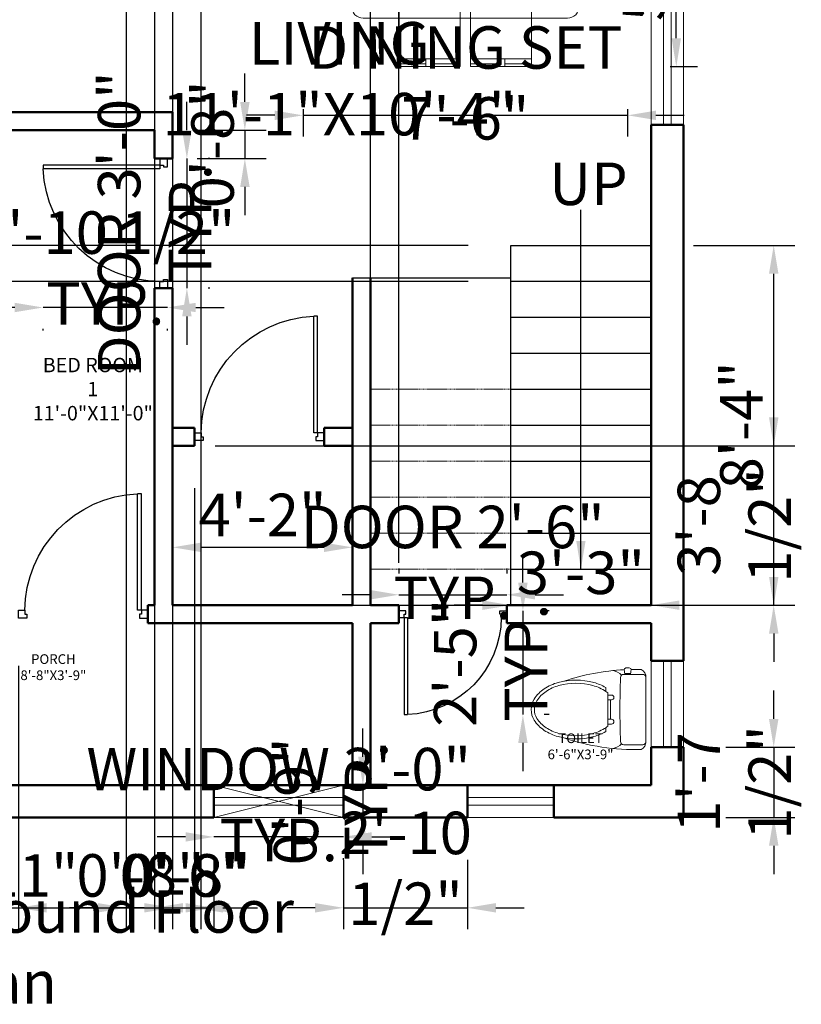
# Model space of a CAD drawing. Units: inches. Extents: x 314 to 688, y 344 to 882.
# Tile 2 of 3: x 471 to 688, y 344 to 618. Entities that reach past the tile are written whole.
import ezdxf

# ---------------------------------------------------------------- set-up
doc = ezdxf.new("R2010")
doc.units = ezdxf.units.IN
doc.header["$MEASUREMENT"] = 0
doc.linetypes.add('HIDDEN', pattern=[0.375, 0.25, -0.125])
for name, color, linetype, lineweight in [('A-ANNO-TEXT', 7, 'Continuous', 25), ('A-AREA-IDEN', 7, 'Continuous', 25), ('A-DOOR', 4, 'Continuous', 25), ('A-FLOR-FIXT', 9, 'Continuous', 18), ('A-FLOR-STRS', 7, 'Continuous', 25), ('A-FLOR-STRS-HIDN', 8, 'HIDDEN', 18), ('A-FURN', 8, 'Continuous', 18), ('WALL', 7, 'Continuous', 50), ('WINDOW', 2, 'Continuous', 18), ('YQ_DIM', 3, 'Continuous', 18)]:
    doc.layers.add(name, color=color, linetype=linetype, lineweight=lineweight)
doc.styles.add('YQ_DIM', font='SUPEROS.SHX', dxfattribs={"width": 0.8, "bigfont": 'HZDX.SHX'})
doc.dimstyles.new('yqi3_937', dxfattribs={"dimscale": 3.937008, "dimtxt": 3, "dimasz": 2, "dimexe": 1.5, "dimexo": 3, "dimgap": 0.5, "dimtad": 1, "dimdsep": 46, "dimlunit": 4, "dimtxsty": 'YQ_DIM', "dimcen": 0, "dimclrd": 256, "dimclre": 256, "dimclrt": 7, "dimadec": 1, "dimazin": 2, "dimtfac": 1, "dimtix": 1, "dimtmove": 2, "dimatfit": 2, "dimfxl": 1, "dimtolj": 1, "dimtzin": 0, "dimarcsym": 0})

# ---------------------------------------------------------------- blocks, each defined once
blk = doc.blocks.new('DR_D01')
for p, q in [((-0.45, 0.93), (-0.42, 0.93)), ((-0.45, 0.03), (-0.45, 0.93)), ((-0.42, 0.03), (-0.42, 0.93)), ((-0.5, 0.03), (-0.42, 0.03)), ((-0.5, 0.03), (-0.5, -0.03)), ((-0.45, 0.03), (-0.45, 0)), ((-0.45, 0), (-0.435, 0)), ((-0.435, 0), (-0.435, -0.03)), ((0.435, 0), (0.435, -0.03)), ((0.45, 0), (0.435, 0)), ((0.45, 0.03), (0.45, 0)), ((0.5, 0.03), (0.45, 0.03)), ((0.5, -0.03), (0.5, 0.03)), ((-0.435, -0.03), (-0.5, -0.03)), ((0.435, -0.03), (0.5, -0.03))]:
    blk.add_line(p, q)
blk.add_arc((-0.4602, 0.0206), 0.9103, 0.59152, 87.46644)
blk = doc.blocks.new('WD_WIN4')
for p, q in [((-0.5, 0.5), (0.5, 0.5)), ((-0.5, 0.12), (0.5, 0.12)), ((-0.5, -0.12), (0.5, -0.12)), ((-0.5, -0.5), (0.5, -0.5))]:
    blk.add_line(p, q)
blk = doc.blocks.new('*D7')
at = {"layer": 'Defpoints', "color": 0, "transparency": 16777216}
for p in [(513.29, 472.16), (563.29, 472.16), (563.29, 471.31)]:
    blk.add_point(p, dxfattribs=at)
at = {"layer": 'YQ_DIM', "color": 0, "lineweight": -2, "transparency": 16777216}
for p, q in [((521.17, 471.31), (555.42, 471.31)), ((513.29, 460.35), (513.29, 465.4)), ((563.29, 460.35), (563.29, 465.4))]:
    blk.add_line(p, q, dxfattribs=at)
at = {"layer": 'YQ_DIM', "color": 0, "transparency": 16777216}
for points in [[(521.17, 472.62), (521.17, 470), (513.29, 471.31)], [(555.42, 472.62), (555.42, 470), (563.29, 471.31)]]:
    blk.add_solid(points, dxfattribs=at)
at = {"layer": 'YQ_DIM', "color": 0, "transparency": 16777216, "insert": (538.29, 480.31), "char_height": 11.811, "attachment_point": 5, "style": 'YQ_DIM'}
blk.add_mtext('\\A1;4\'-2"', dxfattribs=at)
blk = doc.blocks.new('*D9')
at = {"layer": 'Defpoints', "color": 0, "transparency": 16777216}
for p in [(607.29, 460.65), (646.29, 460.65), (646.29, 455.23)]:
    blk.add_point(p, dxfattribs=at)
at = {"layer": 'YQ_DIM', "color": 0, "lineweight": -2, "transparency": 16777216}
for p, q in [((599.42, 455.23), (591.55, 455.23)), ((607.29, 455.23), (646.29, 455.23)), ((654.17, 455.23), (662.04, 455.23)), ((607.29, 448.84), (607.29, 449.33)), ((646.29, 448.84), (646.29, 449.33))]:
    blk.add_line(p, q, dxfattribs=at)
at = {"layer": 'YQ_DIM', "color": 0, "transparency": 16777216}
for points in [[(599.42, 456.54), (599.42, 453.92), (607.29, 455.23)], [(654.17, 456.54), (654.17, 453.92), (646.29, 455.23)]]:
    blk.add_solid(points, dxfattribs=at)
at = {"layer": 'YQ_DIM', "color": 0, "transparency": 16777216, "insert": (626.79, 464.23), "char_height": 11.811, "attachment_point": 5, "style": 'YQ_DIM'}
blk.add_mtext('\\A1;3\'-3"', dxfattribs=at)
blk = doc.blocks.new('yq_matong_01')
for p, q in [((0, 200.5), (0, -200.5)), ((20, 220.5), (138.8, 220.5)), ((252.5, 138), (252.5, 114.5)), ((215.8, 91), (238, 91)), ((238, 104.1), (238, -104.1)), ((215.8, 61), (238, 61)), ((223, 61), (223, -61)), ((215.8, -61), (238, -61)), ((215.8, -91), (238, -91)), ((252.5, -114.5), (252.5, -138)), ((20, -220.5), (138.8, -220.5)), ((97.4, -220.5), (97.4, -225.5)), ((97.4, -225.5), (131.6, -225.5)), ((131.6, -220.5), (131.6, -225.5))]:
    blk.add_line(p, q)
for centre, radius, start, end in [((54.8, 202.4), 54.8, 117.32201, 181.89921), ((63.9, -1165.4), 1416.8, 71.40679, 91.38565), ((20, 200.5), 20, 90, 180), ((138.8, 200.5), 20, 2.30634, 90), ((216.6, 161.2), 83.2, 95.49628, 139.93242), ((-4840.4, 0), 5003.3, 357.69366, 2.30634), ((406.6, -122.9), 283, 105.20877, 123.27785), ((406.6, -122.9), 303, 105.20877, 120.56985), ((439, -242.2), 426.7, 74.79123, 105.20877), ((439, -242.2), 406.7, 74.79123, 105.20877), ((471.4, -122.9), 283, 56.72215, 74.79123), ((471.4, -122.9), 303, 56.72215, 74.79123), ((520.9, -47.5), 212.8, 32.25649, 56.72215), ((215.8, 76), 15, 90, 270), ((357.1, -47.5), 192.8, 123.27785, 128.13838), ((520.9, -47.5), 192.8, 32.25649, 56.72215), ((596.2, 0), 123.8, 360, 32.25649), ((596.2, 0), 103.8, 360, 32.25649), ((215.8, -76), 15, 90, 270), ((520.9, 47.5), 192.8, 303.27785, 327.74351), ((596.2, 0), 103.8, 327.74351, 360), ((596.2, 0), 123.8, 327.74351, 360), ((357.1, 47.5), 192.8, 231.86162, 236.72215), ((406.6, 122.9), 283, 236.72215, 254.79123), ((471.4, 122.9), 283, 285.20877, 303.27785), ((520.9, 47.5), 212.8, 303.27785, 327.74351), ((63.9, 1165.4), 1416.8, 272.89667, 288.59321), ((406.6, 122.9), 303, 239.43015, 254.79123), ((439, 242.2), 426.7, 254.79123, 285.20877), ((439, 242.2), 406.7, 254.79123, 285.20877), ((471.4, 122.9), 303, 285.20877, 303.27785), ((51.3, -204.4), 51.4, 175.68696, 245.09182), ((20, -200.5), 20, 180, 270), ((156.6, -247.4), 63.1, 159.68336, 188.49388), ((72.4, -247.4), 63.1, 352.09441, 20.31664), ((138.8, -200.5), 20, 270, 357.69366), ((216.6, -161.2), 83.2, 220.06758, 264.50372), ((63.9, 1165.4), 1416.8, 268.61435, 271.20362), ((114.1, -225.6), 37, 237.52867, 304.27722)]:
    blk.add_arc(centre, radius, start, end)
blk = doc.blocks.new('East 1200 Sq.ft$0$din1')
for p, q in [((-487.5, 578.6), (-487.5, 807.1)), ((-487.5, 807.1), (-291.1, 807.1)), ((-291.1, 750), (-291.1, 807.1)), ((-291.1, 807.1), (-233.9, 807.1)), ((-233.9, 750), (-233.9, 807.1)), ((-233.9, 807.1), (-37.5, 807.1)), ((-37.5, 807.1), (-37.5, 578.6)), ((37.5, 807.1), (37.5, 578.6)), ((233.9, 807.1), (37.5, 807.1)), ((233.9, 750), (233.9, 807.1)), ((291.1, 807.1), (233.9, 807.1)), ((487.5, 807.1), (291.1, 807.1)), ((291.1, 750), (291.1, 807.1)), ((487.5, 578.6), (487.5, 807.1)), ((-487.5, 785.7), (-291.1, 785.7)), ((-487.5, 750), (-37.5, 750)), ((-233.9, 785.7), (-37.5, 785.7)), ((233.9, 785.7), (37.5, 785.7)), ((487.5, 750), (37.5, 750)), ((487.5, 785.7), (291.1, 785.7)), ((-966.1, 225), (-1194.6, 225)), ((-1194.6, 225), (-1194.6, 28.6)), ((-1173.2, 225), (-1173.2, 28.6)), ((-1137.5, 225), (-1137.5, -225)), ((966.1, 225), (1194.6, 225)), ((1137.5, 225), (1137.5, -225)), ((1173.2, 225), (1173.2, 28.6)), ((1194.6, 225), (1194.6, 28.6)), ((-1137.5, 28.6), (-1194.6, 28.6)), ((-1194.6, 28.6), (-1194.6, -28.6)), ((1137.5, 28.6), (1194.6, 28.6)), ((1194.6, 28.6), (1194.6, -28.6)), ((-1137.5, -28.6), (-1194.6, -28.6)), ((-1194.6, -28.6), (-1194.6, -225)), ((-1173.2, -28.6), (-1173.2, -225)), ((1137.5, -28.6), (1194.6, -28.6)), ((1173.2, -28.6), (1173.2, -225)), ((1194.6, -28.6), (1194.6, -225)), ((-1194.6, -225), (-966.1, -225)), ((1194.6, -225), (966.1, -225)), ((-487.5, -578.6), (-487.5, -807.1)), ((-37.5, -807.1), (-37.5, -578.6)), ((37.5, -807.1), (37.5, -578.6)), ((487.5, -578.6), (487.5, -807.1)), ((-487.5, -750), (-37.5, -750)), ((-487.5, -785.7), (-291.1, -785.7)), ((-291.1, -750), (-291.1, -807.1)), ((-233.9, -750), (-233.9, -807.1)), ((-233.9, -785.7), (-37.5, -785.7)), ((487.5, -750), (37.5, -750)), ((233.9, -785.7), (37.5, -785.7)), ((233.9, -750), (233.9, -807.1)), ((291.1, -750), (291.1, -807.1)), ((487.5, -785.7), (291.1, -785.7)), ((-487.5, -807.1), (-291.1, -807.1)), ((-291.1, -807.1), (-233.9, -807.1)), ((-233.9, -807.1), (-37.5, -807.1)), ((233.9, -807.1), (37.5, -807.1)), ((291.1, -807.1), (233.9, -807.1)), ((487.5, -807.1), (291.1, -807.1))]:
    blk.add_line(p, q)
for points in [[(-37.5, 578.6), (-37.5, 342.9, -0.414214), (-80.4, 300), (-444.6, 300, -0.414214), (-487.5, 342.9), (-487.5, 578.6)], [(37.5, 578.6), (37.5, 342.9, 0.414214), (80.4, 300), (444.6, 300, 0.414214), (487.5, 342.9), (487.5, 578.6)], [(-966.1, -225), (-730.4, -225, 0.414214), (-687.5, -182.1), (-687.5, 182.1, 0.414214), (-730.4, 225), (-966.1, 225)], [(966.1, -225), (730.4, -225, -0.414214), (687.5, -182.1), (687.5, 182.1, -0.414214), (730.4, 225), (966.1, 225)], [(-37.5, -578.6), (-37.5, -342.9, 0.414214), (-80.4, -300), (-444.6, -300, 0.414214), (-487.5, -342.9), (-487.5, -578.6)], [(37.5, -578.6), (37.5, -342.9, -0.414214), (80.4, -300), (444.6, -300, -0.414214), (487.5, -342.9), (487.5, -578.6)]]:
    blk.add_lwpolyline(points, format="xyb")
blk.add_lwpolyline([(751.8, -450), (-751.8, -450, -0.414214), (-837.5, -364.3), (-837.5, 364.3, -0.414214), (-751.8, 450), (751.8, 450, -0.414214), (837.5, 364.3), (837.5, -364.3, -0.414214)], format="xyb", close=True)
blk = doc.blocks.new('*D20')
at = {"layer": 'Defpoints', "color": 0, "transparency": 16777216}
for p in [(524.79, 396.23), (560.79, 396.23), (524.79, 390.83)]:
    blk.add_point(p, dxfattribs=at)
at = {"layer": 'YQ_DIM', "lineweight": -2, "transparency": 16777216}
for p, q in [((516.92, 390.83), (509.05, 390.83)), ((560.79, 390.83), (524.79, 390.83)), ((568.67, 390.83), (576.54, 390.83)), ((524.79, 384.42), (524.79, 384.93)), ((560.79, 384.42), (560.79, 384.93))]:
    blk.add_line(p, q, dxfattribs=at)
at = {"layer": 'YQ_DIM', "transparency": 16777216}
for points in [[(516.92, 392.14), (516.92, 389.52), (524.79, 390.83)], [(568.67, 392.14), (568.67, 389.52), (560.79, 390.83)]]:
    blk.add_solid(points, dxfattribs=at)
at = {"layer": 'YQ_DIM', "color": 7, "transparency": 16777216, "insert": (542.79, 399.83), "char_height": 11.811, "attachment_point": 5, "style": 'YQ_DIM'}
blk.add_mtext('\\A1;WINDOW 3\'-0" TYP.', dxfattribs=at)
blk = doc.blocks.new('*D21')
at = {"layer": 'Defpoints', "color": 0, "transparency": 16777216}
for p in [(560.79, 405.23), (560.79, 396.23), (566.19, 396.23)]:
    blk.add_point(p, dxfattribs=at)
at = {"layer": 'YQ_DIM', "lineweight": -2, "transparency": 16777216}
for p, q in [((566.19, 413.11), (566.19, 420.98)), ((566.19, 405.23), (566.19, 396.23)), ((572.6, 405.23), (572.1, 405.23)), ((572.6, 396.23), (572.1, 396.23)), ((566.19, 388.36), (566.19, 380.48))]:
    blk.add_line(p, q, dxfattribs=at)
at = {"layer": 'YQ_DIM', "transparency": 16777216}
for points in [[(564.88, 413.11), (567.51, 413.11), (566.19, 405.23)], [(564.88, 388.36), (567.51, 388.36), (566.19, 396.23)]]:
    blk.add_solid(points, dxfattribs=at)
at = {"layer": 'YQ_DIM', "color": 7, "transparency": 16777216, "insert": (557.2, 400.73), "char_height": 11.811, "attachment_point": 5, "rotation": 90, "style": 'YQ_DIM'}
blk.add_mtext('\\A1;0\'-9" TYP.', dxfattribs=at)
blk = doc.blocks.new('*D22')
at = {"layer": 'Defpoints', "color": 0, "transparency": 16777216}
for p in [(606.17, 458.13), (576.17, 453.63), (606.17, 453.63)]:
    blk.add_point(p, dxfattribs=at)
at = {"layer": 'YQ_DIM', "lineweight": -2, "transparency": 16777216}
for p, q in [((576.17, 465.44), (576.17, 464.04)), ((606.17, 465.44), (606.17, 464.04)), ((568.29, 458.13), (560.42, 458.13)), ((576.17, 458.13), (606.17, 458.13)), ((614.04, 458.13), (621.92, 458.13))]:
    blk.add_line(p, q, dxfattribs=at)
at = {"layer": 'YQ_DIM', "transparency": 16777216}
for points in [[(568.29, 459.44), (568.29, 456.82), (576.17, 458.13)], [(614.04, 459.44), (614.04, 456.82), (606.17, 458.13)]]:
    blk.add_solid(points, dxfattribs=at)
at = {"layer": 'YQ_DIM', "color": 7, "transparency": 16777216, "insert": (591.17, 467.13), "char_height": 11.811, "attachment_point": 5, "style": 'YQ_DIM'}
blk.add_mtext('\\A1;DOOR 2\'-6" TYP.', dxfattribs=at)
blk = doc.blocks.new('*D23')
at = {"layer": 'Defpoints', "color": 0, "transparency": 16777216}
for p in [(606.17, 453.63), (606.17, 424.83), (610.67, 424.83)]:
    blk.add_point(p, dxfattribs=at)
at = {"layer": 'YQ_DIM', "lineweight": -2, "transparency": 16777216}
for p, q in [((610.67, 461.51), (610.67, 469.38)), ((610.67, 453.63), (610.67, 424.83)), ((617.98, 453.63), (616.57, 453.63)), ((617.98, 424.83), (616.57, 424.83)), ((610.67, 416.96), (610.67, 409.08))]:
    blk.add_line(p, q, dxfattribs=at)
at = {"layer": 'YQ_DIM', "transparency": 16777216}
for points in [[(609.36, 461.51), (611.98, 461.51), (610.67, 453.63)], [(609.36, 416.96), (611.98, 416.96), (610.67, 424.83)]]:
    blk.add_solid(points, dxfattribs=at)
at = {"layer": 'YQ_DIM', "color": 7, "transparency": 16777216, "insert": (601.67, 439.23), "char_height": 11.811, "attachment_point": 5, "rotation": 90, "style": 'YQ_DIM'}
blk.add_mtext('\\A1;2\'-5" TYP.', dxfattribs=at)
blk = doc.blocks.new('*D24')
at = {"layer": 'Defpoints', "color": 0, "transparency": 16777216}
for p in [(511.87, 579.36), (511.87, 543.36), (517.27, 543.36)]:
    blk.add_point(p, dxfattribs=at)
at = {"layer": 'YQ_DIM', "lineweight": -2, "transparency": 16777216}
for p, q in [((517.27, 587.23), (517.27, 595.11)), ((517.27, 579.36), (517.27, 543.36)), ((523.68, 579.36), (523.18, 579.36)), ((523.68, 543.36), (523.18, 543.36)), ((517.27, 535.48), (517.27, 527.61))]:
    blk.add_line(p, q, dxfattribs=at)
at = {"layer": 'YQ_DIM', "transparency": 16777216}
for points in [[(515.96, 587.23), (518.59, 587.23), (517.27, 579.36)], [(515.96, 535.48), (518.59, 535.48), (517.27, 543.36)]]:
    blk.add_solid(points, dxfattribs=at)
at = {"layer": 'YQ_DIM', "color": 7, "transparency": 16777216, "insert": (508.28, 561.36), "char_height": 11.811, "attachment_point": 5, "rotation": 90, "style": 'YQ_DIM'}
blk.add_mtext('\\A1;DOOR 3\'-0" TYP.', dxfattribs=at)
blk = doc.blocks.new('*D25')
at = {"layer": 'Defpoints', "color": 0, "transparency": 16777216}
for p in [(477.31, 543.36), (511.87, 543.36), (477.31, 537.96)]:
    blk.add_point(p, dxfattribs=at)
at = {"layer": 'YQ_DIM', "lineweight": -2, "transparency": 16777216}
for p, q in [((469.44, 537.96), (461.57, 537.96)), ((511.87, 537.96), (477.31, 537.96)), ((519.75, 537.96), (527.62, 537.96)), ((477.31, 531.55), (477.31, 532.05)), ((511.87, 531.55), (511.87, 532.05))]:
    blk.add_line(p, q, dxfattribs=at)
at = {"layer": 'YQ_DIM', "transparency": 16777216}
for points in [[(469.44, 539.27), (469.44, 536.65), (477.31, 537.96)], [(519.75, 539.27), (519.75, 536.65), (511.87, 537.96)]]:
    blk.add_solid(points, dxfattribs=at)
at = {"layer": 'YQ_DIM', "color": 7, "transparency": 16777216, "insert": (494.59, 548.93), "char_height": 11.811, "attachment_point": 5, "style": 'YQ_DIM'}
blk.add_mtext('\\A1;2\'-10 1/2" TYP.', dxfattribs=at)
blk = doc.blocks.new('*D34')
at = {"layer": 'Defpoints', "color": 0, "transparency": 16777216}
for p in [(549.56, 604.9), (639.78, 604.9), (639.78, 591.37)]:
    blk.add_point(p, dxfattribs=at)
at = {"layer": 'YQ_DIM', "lineweight": -2, "transparency": 16777216}
for p, q in [((541.68, 591.37), (533.81, 591.37)), ((549.56, 593.09), (549.56, 585.46)), ((549.56, 591.37), (639.78, 591.37)), ((639.78, 593.09), (639.78, 585.46)), ((647.65, 591.37), (655.53, 591.37))]:
    blk.add_line(p, q, dxfattribs=at)
at = {"layer": 'YQ_DIM', "transparency": 16777216}
for points in [[(541.68, 592.68), (541.68, 590.05), (549.56, 591.37)], [(647.65, 592.68), (647.65, 590.05), (639.78, 591.37)]]:
    blk.add_solid(points, dxfattribs=at)
at = {"layer": 'YQ_DIM', "color": 7, "transparency": 16777216, "insert": (594.67, 600.37), "char_height": 11.811, "attachment_point": 5, "style": 'YQ_DIM'}
blk.add_mtext('\\A1;DINING SET 7\'-6"', dxfattribs=at)
blk = doc.blocks.new('*D35')
at = {"layer": 'Defpoints', "color": 0, "transparency": 16777216}
for p in [(639.78, 665.86), (653.31, 665.86), (639.78, 604.9)]:
    blk.add_point(p, dxfattribs=at)
at = {"layer": 'YQ_DIM', "lineweight": -2, "transparency": 16777216}
for p, q in [((651.59, 665.86), (659.22, 665.86)), ((653.31, 612.77), (653.31, 657.98)), ((651.59, 604.9), (659.22, 604.9))]:
    blk.add_line(p, q, dxfattribs=at)
at = {"layer": 'YQ_DIM', "transparency": 16777216}
for points in [[(652, 657.98), (654.62, 657.98), (653.31, 665.86)], [(652, 612.77), (654.62, 612.77), (653.31, 604.9)]]:
    blk.add_solid(points, dxfattribs=at)
at = {"layer": 'YQ_DIM', "color": 7, "transparency": 16777216, "insert": (644.31, 635.38), "char_height": 11.811, "attachment_point": 5, "rotation": 90, "style": 'YQ_DIM'}
blk.add_mtext('\\A1;5\'-1"', dxfattribs=at)
blk = doc.blocks.new('*D38')
at = {"layer": 'Defpoints', "color": 0, "transparency": 16777216}
for p in [(655.29, 415.73), (655.29, 396.23), (680.39, 396.23)]:
    blk.add_point(p, dxfattribs=at)
at = {"layer": 'YQ_DIM', "lineweight": -2, "transparency": 16777216}
for p, q in [((680.39, 423.61), (680.39, 431.48)), ((667.1, 415.73), (686.3, 415.73)), ((680.39, 415.73), (680.39, 396.23)), ((667.1, 396.23), (686.3, 396.23)), ((680.39, 388.36), (680.39, 380.48))]:
    blk.add_line(p, q, dxfattribs=at)
at = {"layer": 'YQ_DIM', "transparency": 16777216}
for points in [[(679.08, 423.61), (681.71, 423.61), (680.39, 415.73)], [(679.08, 388.36), (681.71, 388.36), (680.39, 396.23)]]:
    blk.add_solid(points, dxfattribs=at)
at = {"layer": 'YQ_DIM', "color": 7, "transparency": 16777216, "insert": (669.43, 405.98), "char_height": 11.811, "attachment_point": 5, "rotation": 90, "style": 'YQ_DIM'}
blk.add_mtext('\\A1;1\'-7 1/2"', dxfattribs=at)
blk = doc.blocks.new('*D39')
at = {"layer": 'Defpoints', "color": 0, "transparency": 16777216}
for p in [(646.29, 555.23), (680.39, 555.23), (646.29, 455.23)]:
    blk.add_point(p, dxfattribs=at)
at = {"layer": 'YQ_DIM', "lineweight": -2, "transparency": 16777216}
for p, q in [((658.1, 555.23), (686.3, 555.23)), ((680.39, 463.11), (680.39, 547.36)), ((658.1, 455.23), (686.3, 455.23))]:
    blk.add_line(p, q, dxfattribs=at)
at = {"layer": 'YQ_DIM', "transparency": 16777216}
for points in [[(679.08, 547.36), (681.71, 547.36), (680.39, 555.23)], [(679.08, 463.11), (681.71, 463.11), (680.39, 455.23)]]:
    blk.add_solid(points, dxfattribs=at)
at = {"layer": 'YQ_DIM', "color": 7, "transparency": 16777216, "insert": (671.4, 505.23), "char_height": 11.811, "attachment_point": 5, "rotation": 90, "style": 'YQ_DIM'}
blk.add_mtext('\\A1;8\'-4"', dxfattribs=at)
blk = doc.blocks.new('*D40')
at = {"layer": 'Defpoints', "color": 0, "transparency": 16777216}
for p in [(342.19, 555.23), (607.29, 555.23), (607.29, 545.23)]:
    blk.add_point(p, dxfattribs=at)
at = {"layer": 'YQ_DIM', "lineweight": -2, "transparency": 16777216}
for p, q in [((342.19, 563.11), (342.19, 570.98)), ((595.48, 555.23), (336.29, 555.23)), ((342.19, 545.23), (342.19, 555.23)), ((595.48, 545.23), (336.29, 545.23)), ((342.19, 537.36), (342.19, 529.48))]:
    blk.add_line(p, q, dxfattribs=at)
at = {"layer": 'YQ_DIM', "transparency": 16777216}
for points in [[(340.88, 563.11), (343.51, 563.11), (342.19, 555.23)], [(340.88, 537.36), (343.51, 537.36), (342.19, 545.23)]]:
    blk.add_solid(points, dxfattribs=at)
at = {"layer": 'YQ_DIM', "color": 7, "transparency": 16777216, "insert": (333.2, 550.23), "char_height": 11.811, "attachment_point": 5, "rotation": 90, "style": 'YQ_DIM'}
blk.add_mtext('\\A1;0\'-10"', dxfattribs=at)
blk = doc.blocks.new('*D46')
at = {"layer": 'Defpoints', "color": 0, "transparency": 16777216}
for p in [(367.29, 396.23), (524.79, 396.23), (524.79, 371.13)]:
    blk.add_point(p, dxfattribs=at)
at = {"layer": 'YQ_DIM', "lineweight": -2, "transparency": 16777216}
for p, q in [((367.29, 384.42), (367.29, 365.23)), ((524.79, 384.42), (524.79, 365.23)), ((375.17, 371.13), (516.92, 371.13))]:
    blk.add_line(p, q, dxfattribs=at)
at = {"layer": 'YQ_DIM', "transparency": 16777216}
for points in [[(375.17, 372.44), (375.17, 369.82), (367.29, 371.13)], [(516.92, 372.44), (516.92, 369.82), (524.79, 371.13)]]:
    blk.add_solid(points, dxfattribs=at)
at = {"layer": 'YQ_DIM', "color": 7, "transparency": 16777216, "insert": (446.04, 382.1), "char_height": 11.811, "attachment_point": 5, "style": 'YQ_DIM'}
blk.add_mtext('\\A1;13\'-1 1/2"', dxfattribs=at)
blk = doc.blocks.new('*D47')
at = {"layer": 'Defpoints', "color": 0, "transparency": 16777216}
for p in [(560.79, 396.23), (595.29, 396.23), (595.29, 371.13)]:
    blk.add_point(p, dxfattribs=at)
at = {"layer": 'YQ_DIM', "lineweight": -2, "transparency": 16777216}
for p, q in [((560.79, 384.42), (560.79, 365.23)), ((595.29, 384.42), (595.29, 365.23)), ((552.92, 371.13), (545.05, 371.13)), ((560.79, 371.13), (595.29, 371.13)), ((603.17, 371.13), (611.04, 371.13))]:
    blk.add_line(p, q, dxfattribs=at)
at = {"layer": 'YQ_DIM', "transparency": 16777216}
for points in [[(552.92, 372.44), (552.92, 369.82), (560.79, 371.13)], [(603.17, 372.44), (603.17, 369.82), (595.29, 371.13)]]:
    blk.add_solid(points, dxfattribs=at)
at = {"layer": 'YQ_DIM', "color": 7, "transparency": 16777216, "insert": (578.04, 382.1), "char_height": 11.811, "attachment_point": 5, "style": 'YQ_DIM'}
blk.add_mtext('\\A1;2\'-10 1/2"', dxfattribs=at)
blk = doc.blocks.new('*D48')
at = {"layer": 'Defpoints', "color": 0, "transparency": 16777216}
for p in [(513.29, 499.55), (680.39, 499.55), (513.29, 455.23)]:
    blk.add_point(p, dxfattribs=at)
at = {"layer": 'YQ_DIM', "lineweight": -2, "transparency": 16777216}
for p, q in [((680.39, 507.42), (680.39, 515.3)), ((525.1, 499.55), (686.3, 499.55)), ((680.39, 455.23), (680.39, 499.55)), ((525.1, 455.23), (686.3, 455.23)), ((680.39, 447.36), (680.39, 439.48))]:
    blk.add_line(p, q, dxfattribs=at)
at = {"layer": 'YQ_DIM', "transparency": 16777216}
for points in [[(679.08, 507.42), (681.71, 507.42), (680.39, 499.55)], [(679.08, 447.36), (681.71, 447.36), (680.39, 455.23)]]:
    blk.add_solid(points, dxfattribs=at)
at = {"layer": 'YQ_DIM', "color": 7, "transparency": 16777216, "insert": (669.43, 477.39), "char_height": 11.811, "attachment_point": 5, "rotation": 90, "style": 'YQ_DIM'}
blk.add_mtext('\\A1;3\'-8 1/2"', dxfattribs=at)
blk = doc.blocks.new('*D49')
at = {"layer": 'Defpoints', "color": 0, "transparency": 16777216}
for p in [(508.29, 675.23), (500.42, 670.23), (508.29, 371.13)]:
    blk.add_point(p, dxfattribs=at)
at = {"layer": 'YQ_DIM', "lineweight": -2, "transparency": 16777216}
for p, q in [((508.29, 663.42), (508.29, 365.23)), ((500.42, 658.42), (500.42, 365.23)), ((492.55, 371.13), (484.67, 371.13)), ((500.42, 371.13), (508.29, 371.13)), ((516.17, 371.13), (524.04, 371.13))]:
    blk.add_line(p, q, dxfattribs=at)
at = {"layer": 'YQ_DIM', "transparency": 16777216}
for points in [[(492.55, 372.44), (492.55, 369.82), (500.42, 371.13)], [(516.17, 372.44), (516.17, 369.82), (508.29, 371.13)]]:
    blk.add_solid(points, dxfattribs=at)
at = {"layer": 'YQ_DIM', "color": 7, "transparency": 16777216, "insert": (504.36, 380.13), "char_height": 11.811, "attachment_point": 5, "style": 'YQ_DIM'}
blk.add_mtext('\\A1;0\'-8"', dxfattribs=at)
blk = doc.blocks.new('*D50')
at = {"layer": 'Defpoints', "color": 0, "transparency": 16777216}
for p in [(513.29, 675.23), (521.17, 670.23), (521.17, 371.13)]:
    blk.add_point(p, dxfattribs=at)
at = {"layer": 'YQ_DIM', "lineweight": -2, "transparency": 16777216}
for p, q in [((513.29, 663.42), (513.29, 365.23)), ((521.17, 658.42), (521.17, 365.23)), ((505.42, 371.13), (497.55, 371.13)), ((513.29, 371.13), (521.17, 371.13)), ((529.04, 371.13), (536.92, 371.13))]:
    blk.add_line(p, q, dxfattribs=at)
at = {"layer": 'YQ_DIM', "transparency": 16777216}
for points in [[(505.42, 372.44), (505.42, 369.82), (513.29, 371.13)], [(529.04, 372.44), (529.04, 369.82), (521.17, 371.13)]]:
    blk.add_solid(points, dxfattribs=at)
at = {"layer": 'YQ_DIM', "color": 7, "transparency": 16777216, "insert": (517.23, 380.13), "char_height": 11.811, "attachment_point": 5, "style": 'YQ_DIM'}
blk.add_mtext('\\A1;0\'-8"', dxfattribs=at)
blk = doc.blocks.new('*D51')
at = {"layer": 'Defpoints', "color": 0, "transparency": 16777216}
for p in [(508.29, 587.23), (508.29, 579.36), (533.39, 579.36)]:
    blk.add_point(p, dxfattribs=at)
at = {"layer": 'YQ_DIM', "lineweight": -2, "transparency": 16777216}
for p, q in [((533.39, 595.11), (533.39, 602.98)), ((520.1, 587.23), (539.3, 587.23)), ((533.39, 587.23), (533.39, 579.36)), ((520.1, 579.36), (539.3, 579.36)), ((533.39, 571.48), (533.39, 563.61))]:
    blk.add_line(p, q, dxfattribs=at)
at = {"layer": 'YQ_DIM', "transparency": 16777216}
for points in [[(532.08, 595.11), (534.71, 595.11), (533.39, 587.23)], [(532.08, 571.48), (534.71, 571.48), (533.39, 579.36)]]:
    blk.add_solid(points, dxfattribs=at)
at = {"layer": 'YQ_DIM', "color": 7, "transparency": 16777216, "insert": (524.4, 583.3), "char_height": 11.811, "attachment_point": 5, "rotation": 90, "style": 'YQ_DIM'}
blk.add_mtext('\\A1;0\'-8"', dxfattribs=at)
blk = doc.blocks.new('*D52')
at = {"layer": 'Defpoints', "color": 0, "transparency": 16777216}
for p in [(576.17, 865.33), (568.29, 455.23), (576.17, 455.23)]:
    blk.add_point(p, dxfattribs=at)
at = {"layer": 'YQ_DIM', "lineweight": -2, "transparency": 16777216}
for p, q in [((568.29, 467.04), (568.29, 871.24)), ((576.17, 467.04), (576.17, 871.24)), ((560.42, 865.33), (552.55, 865.33)), ((568.29, 865.33), (576.17, 865.33)), ((584.04, 865.33), (591.92, 865.33))]:
    blk.add_line(p, q, dxfattribs=at)
at = {"layer": 'YQ_DIM', "transparency": 16777216}
for points in [[(560.42, 866.64), (560.42, 864.02), (568.29, 865.33)], [(584.04, 866.64), (584.04, 864.02), (576.17, 865.33)]]:
    blk.add_solid(points, dxfattribs=at)
at = {"layer": 'YQ_DIM', "color": 7, "transparency": 16777216, "insert": (572.23, 874.33), "char_height": 11.811, "attachment_point": 5, "style": 'YQ_DIM'}
blk.add_mtext('\\A1;0\'-8"', dxfattribs=at)
blk = doc.blocks.new('*D53')
at = {"layer": 'Defpoints', "color": 0, "transparency": 16777216}
for p in [(459.29, 450.23), (470.42, 450.23), (470.42, 371.13)]:
    blk.add_point(p, dxfattribs=at)
at = {"layer": 'YQ_DIM', "lineweight": -2, "transparency": 16777216}
for p, q in [((459.29, 438.42), (459.29, 365.23)), ((470.42, 438.42), (470.42, 365.23)), ((451.42, 371.13), (443.55, 371.13)), ((459.29, 371.13), (470.42, 371.13)), ((478.29, 371.13), (486.17, 371.13))]:
    blk.add_line(p, q, dxfattribs=at)
at = {"layer": 'YQ_DIM', "transparency": 16777216}
for points in [[(451.42, 372.44), (451.42, 369.82), (459.29, 371.13)], [(478.29, 372.44), (478.29, 369.82), (470.42, 371.13)]]:
    blk.add_solid(points, dxfattribs=at)
at = {"layer": 'YQ_DIM', "color": 7, "transparency": 16777216, "insert": (464.86, 380.13), "char_height": 11.811, "attachment_point": 5, "style": 'YQ_DIM'}
blk.add_mtext('\\A1;0\'-11"', dxfattribs=at)
blk = doc.blocks.new('*D54')
at = {"layer": 'Defpoints', "color": 0, "transparency": 16777216}
for p in [(513.29, 499.55), (519.42, 499.55), (519.42, 371.13)]:
    blk.add_point(p, dxfattribs=at)
at = {"layer": 'YQ_DIM', "lineweight": -2, "transparency": 16777216}
for p, q in [((513.29, 487.74), (513.29, 365.23)), ((519.42, 487.74), (519.42, 365.23)), ((505.42, 371.13), (497.55, 371.13)), ((513.29, 371.13), (519.42, 371.13)), ((527.29, 371.13), (535.17, 371.13))]:
    blk.add_line(p, q, dxfattribs=at)
at = {"layer": 'YQ_DIM', "transparency": 16777216}
for points in [[(505.42, 372.44), (505.42, 369.82), (513.29, 371.13)], [(527.29, 372.44), (527.29, 369.82), (519.42, 371.13)]]:
    blk.add_solid(points, dxfattribs=at)
at = {"layer": 'YQ_DIM', "color": 7, "transparency": 16777216, "insert": (516.36, 380.13), "char_height": 11.811, "attachment_point": 5, "style": 'YQ_DIM'}
blk.add_mtext('\\A1;0\'-6"', dxfattribs=at)

msp = doc.modelspace()

# ---------------------------------------------------------------- linework, layer by layer
at = {"layer": 'A-FLOR-STRS'}
for p, q in [((607.294, 455.233), (607.294, 555.233)), ((607.294, 555.233), (646.294, 555.233)), ((563.294, 546.233), (607.294, 546.233)), ((607.294, 545.233), (646.294, 545.233)), ((607.294, 535.233), (646.294, 535.233)), ((607.294, 525.233), (646.294, 525.233)), ((607.294, 515.233), (646.294, 515.233)), ((607.294, 505.233), (646.294, 505.233)), ((607.294, 495.233), (646.294, 495.233)), ((607.294, 485.233), (646.294, 485.233)), ((607.294, 475.233), (646.294, 475.233)), ((607.294, 465.233), (646.294, 465.233))]:
    msp.add_line(p, q, dxfattribs=at)
at = {"layer": 'A-FLOR-STRS-HIDN'}
for p, q in [((568.294, 515.233), (607.294, 515.233)), ((568.294, 505.233), (607.294, 505.233)), ((568.294, 495.233), (607.294, 495.233)), ((568.294, 485.233), (607.294, 485.233)), ((568.294, 475.233), (607.294, 475.233)), ((568.294, 465.233), (607.294, 465.233))]:
    msp.add_line(p, q, dxfattribs=at)
at = {"layer": 'WALL'}
for p, q in [((376.294, 592.233), (513.294, 592.233)), ((513.294, 579.359), (513.294, 592.233)), ((646.294, 455.233), (646.294, 588.733)), ((646.294, 588.733), (655.294, 588.733)), ((655.294, 439.733), (655.294, 588.733)), ((376.294, 587.233), (508.294, 587.233)), ((508.294, 579.359), (508.294, 587.233)), ((508.294, 579.359), (513.294, 579.359)), ((563.294, 455.233), (563.294, 546.233)), ((568.294, 455.233), (568.294, 546.233)), ((508.294, 455.233), (508.294, 543.359)), ((513.294, 543.359), (508.294, 543.359)), ((513.294, 455.233), (513.294, 543.359)), ((513.294, 504.55), (519.42, 504.55)), ((519.42, 499.55), (519.42, 504.55)), ((555.42, 504.55), (563.294, 504.55)), ((555.42, 499.55), (555.42, 504.55)), ((513.294, 499.55), (519.42, 499.55)), ((555.42, 499.55), (563.294, 499.55)), ((506.42, 455.233), (508.294, 455.233)), ((506.42, 450.233), (506.42, 455.233)), ((513.294, 455.233), (563.294, 455.233)), ((568.294, 455.233), (576.168, 455.233)), ((576.168, 450.233), (576.168, 455.233)), ((606.168, 455.233), (607.294, 455.233)), ((606.168, 450.233), (606.168, 455.233)), ((607.294, 455.233), (646.294, 455.233)), ((506.42, 450.233), (563.294, 450.233)), ((563.294, 450.233), (563.294, 405.233)), ((568.294, 450.233), (568.294, 405.233)), ((568.294, 450.233), (576.168, 450.233)), ((606.168, 450.233), (646.294, 450.233)), ((646.294, 439.733), (646.294, 450.233)), ((646.294, 439.733), (655.294, 439.733)), ((646.294, 405.233), (646.294, 415.733)), ((646.294, 415.733), (655.294, 415.733)), ((655.294, 396.233), (655.294, 415.733)), ((459.294, 405.233), (563.294, 405.233)), ((522.294, 405.233), (524.794, 405.233)), ((524.794, 405.233), (524.794, 396.233)), ((560.794, 405.233), (563.294, 405.233)), ((560.794, 405.233), (560.794, 396.233)), ((568.294, 405.233), (595.294, 405.233)), ((568.294, 405.233), (646.294, 405.233)), ((595.294, 405.233), (595.294, 396.233)), ((619.294, 405.233), (646.294, 405.233)), ((619.294, 405.233), (619.294, 396.233)), ((367.294, 396.233), (524.794, 396.233)), ((560.794, 396.233), (595.294, 396.233)), ((619.294, 396.233), (655.294, 396.233))]:
    msp.add_line(p, q, dxfattribs=at)
at = {"layer": 'WINDOW'}
for p, q in [((560.794, 405.233), (524.794, 396.233)), ((524.794, 396.233), (524.794, 405.233)), ((524.794, 405.233), (560.794, 396.233))]:
    msp.add_line(p, q, dxfattribs=at)

# ---------------------------------------------------------------- block references
at = {"layer": 'A-DOOR'}
for p, xscale, yscale, zscale, rotation in [((510.794, 561.359), 36, -36, 36, 270), ((537.42, 502.05), 36, -36, 36, 179.9999999999999), ((591.168, 452.733), 30, -30, 30, 359.9999999999999)]:
    msp.add_blockref('DR_D01', p, dxfattribs=dict(at, xscale=xscale, yscale=yscale, zscale=zscale, rotation=rotation))
at = {"layer": 'A-DOOR', "xscale": -36, "yscale": 36, "zscale": 36}
msp.add_blockref('DR_D01', (488.42, 452.733), dxfattribs=at)
at = {"layer": 'A-FLOR-FIXT', "xscale": 0.0443114336064022, "yscale": 0.0443114336064022, "zscale": 0.0443114336064022, "rotation": 180}
msp.add_blockref('yq_matong_01', (644.869, 426.23), dxfattribs=at)
at = {"layer": 'A-FURN', "xscale": 0.0377605260580774, "yscale": 0.0377605260580774, "zscale": 0.0377605260580774}
msp.add_blockref('East 1200 Sq.ft$0$din1', (594.669, 635.378), dxfattribs=at)
at = {"layer": 'WINDOW'}
for p, xscale, yscale, zscale, rotation in [((650.794, 612.733), 48, 9.000000000001476, 48, 269.9999999999998), ((650.794, 427.733), 24, 9.000000000000227, 24, 269.9999999999998), ((542.794, 400.733), 36, 9.000000000001876, 36, 179.9999999999996), ((607.294, 400.733), 24, 9.000000000002387, 24, 179.9999999999996)]:
    msp.add_blockref('WD_WIN4', p, dxfattribs=dict(at, xscale=xscale, yscale=yscale, zscale=zscale, rotation=rotation))

# ---------------------------------------------------------------- texts
at = {"layer": 'A-ANNO-TEXT', "attachment_point": 1, "style": 'YQ_DIM'}
for s, insert, char_height, width in [('\\pxqc;UP', (620.065, 578.245), 11.811, 17.64326), ('Ground Floor Plan', (447.466, 376.019), 11.81102, 110.27862)]:
    msp.add_mtext(s, dxfattribs=dict(at, insert=insert, char_height=char_height, width=width))
at = {"layer": 'A-AREA-IDEN', "attachment_point": 1, "style": 'YQ_DIM'}
for s, insert, char_height, width in [('\\pxqc;LIVING\\P11\'-1"X10\'-4"', (513.294, 617.292), 11.81102, 92.67922), ('\\pxqc;BED ROOM 1\\P11\'-0"X11\'-0"', (475.397, 523.972), 4.01009, 31.46653), ('\\pxqc;PORCH\\P8\'-8"X3\'-9"', (469.604, 441.595), 2.69012, 21.10895), ('\\pxqc;TOILET\\P6\'-6"X3\'-9"', (616.138, 419.596), 2.69012, 21.10895)]:
    msp.add_mtext(s, dxfattribs=dict(at, insert=insert, char_height=char_height, width=width))

# ---------------------------------------------------------------- dimensions: what is measured, and where the dimension line sits
at = {"layer": 'YQ_DIM'}
for base, p1, p2, picture, middle in [((576.168, 865.333), (568.294, 455.233), (576.168, 455.233), '*D52', (572.231, 874.331)), ((508.294, 371.133), (500.42, 670.233), (508.294, 675.233), '*D49', (504.357, 380.131)), ((521.168, 371.133), (513.294, 675.233), (521.168, 670.233), '*D50', (517.231, 380.131)), ((519.42, 371.133), (513.294, 499.55), (519.42, 499.55), '*D54', (516.357, 380.131)), ((470.42, 371.133), (459.294, 450.233), (470.42, 450.233), '*D53', (464.857, 380.131)), ((524.794, 371.133), (367.294, 396.233), (524.794, 396.233), '*D46', (446.044, 382.1)), ((595.294, 371.133), (560.794, 396.233), (595.294, 396.233), '*D47', (578.044, 382.1))]:
    dim = msp.add_linear_dim(base=base, p1=p1, p2=p2, dimstyle='yqi3_937', override={"dimdec": 1, "dimlfac": 1, "dimrnd": 0, "dimzin": 1, "dimdsep": 46, "dimlunit": 4, "dimfrac": 2}, dxfattribs=at)
    dim.commit()
    dim.dimension.update_dxf_attribs({"geometry": picture, "text_midpoint": middle})
for base, p1, p2, angle, picture, middle in [((653.313, 665.856), (639.779, 604.899), (639.779, 665.856), 90, '*D35', (644.314, 635.378)), ((533.394, 579.359), (508.294, 587.233), (508.294, 579.359), 270, '*D51', (524.395, 583.296)), ((342.194, 555.233), (607.294, 545.233), (607.294, 555.233), 90, '*D40', (333.195, 550.233)), ((680.394, 555.233), (646.294, 455.233), (646.294, 555.233), 90, '*D39', (671.395, 505.233)), ((680.394, 499.55), (513.294, 455.233), (513.294, 499.55), 90, '*D48', (669.427, 477.391)), ((680.394, 396.233), (655.294, 415.733), (655.294, 396.233), 90, '*D38', (669.427, 405.983))]:
    dim = msp.add_linear_dim(base=base, p1=p1, p2=p2, angle=angle, dimstyle='yqi3_937', override={"dimdec": 1, "dimlfac": 1, "dimrnd": 0, "dimzin": 1, "dimdsep": 46, "dimlunit": 4, "dimfrac": 2}, dxfattribs=at)
    dim.commit()
    dim.dimension.update_dxf_attribs({"geometry": picture, "text_midpoint": middle})
for base, p1, p2, text, picture, middle in [((639.779, 591.366), (549.559, 604.899), (639.779, 604.899), 'DINING SET <>', '*D34', (594.669, 600.365)), ((606.168, 458.133), (576.168, 453.633), (606.168, 453.633), 'DOOR <> TYP.', '*D22', (591.168, 467.131))]:
    dim = msp.add_linear_dim(base=base, p1=p1, p2=p2, text=text, dimstyle='yqi3_937', override={"dimdec": 1, "dimlfac": 1, "dimrnd": 0, "dimzin": 1, "dimdsep": 46, "dimlunit": 4, "dimfrac": 2}, dxfattribs=at)
    dim.commit()
    dim.dimension.update_dxf_attribs({"geometry": picture, "text_midpoint": middle})
for base, p1, p2, angle, text, picture, middle in [((517.274, 543.359), (511.874, 579.359), (511.874, 543.359), 270, 'DOOR <> TYP.', '*D24', (508.275, 561.359)), ((477.314, 537.959), (511.874, 543.359), (477.314, 543.359), 180, '<> TYP.', '*D25', (494.594, 548.926)), ((610.668, 424.833), (606.168, 453.633), (606.168, 424.833), 270, '<> TYP.', '*D23', (601.669, 439.233)), ((524.794, 390.833), (560.794, 396.233), (524.794, 396.233), 180, 'WINDOW <> TYP.', '*D20', (542.794, 399.831)), ((566.194, 396.233), (560.794, 405.233), (560.794, 396.233), 270, '<> TYP.', '*D21', (557.195, 400.733))]:
    dim = msp.add_linear_dim(base=base, p1=p1, p2=p2, angle=angle, text=text, dimstyle='yqi3_937', override={"dimdec": 1, "dimlfac": 1, "dimrnd": 0, "dimzin": 1, "dimdsep": 46, "dimlunit": 4, "dimfrac": 2}, dxfattribs=at)
    dim.commit()
    dim.dimension.update_dxf_attribs({"geometry": picture, "text_midpoint": middle})
for p1, p2, distance, picture, middle in [((513.294, 472.165), (563.294, 472.165), -0.856, '*D7', (538.294, 480.307)), ((607.294, 460.649), (646.294, 460.649), -5.416, '*D9', (626.794, 464.231))]:
    dim = msp.add_aligned_dim(p1=p1, p2=p2, distance=distance, dimstyle='yqi3_937', override={"dimclrd": 0, "dimclre": 0, "dimclrt": 0}, dxfattribs=at)
    dim.commit()
    dim.dimension.update_dxf_attribs({"geometry": picture, "text_midpoint": middle})

# ---------------------------------------------------------------- leaders
at = {"layer": 'A-FLOR-STRS'}
msp.add_leader([(626.794, 465.233), (626.794, 565.145)], dimstyle='yqi3_937', override={"dimgap": 0.5, "dimtad": 0}, dxfattribs=at)

doc.saveas('drawing.dxf')
